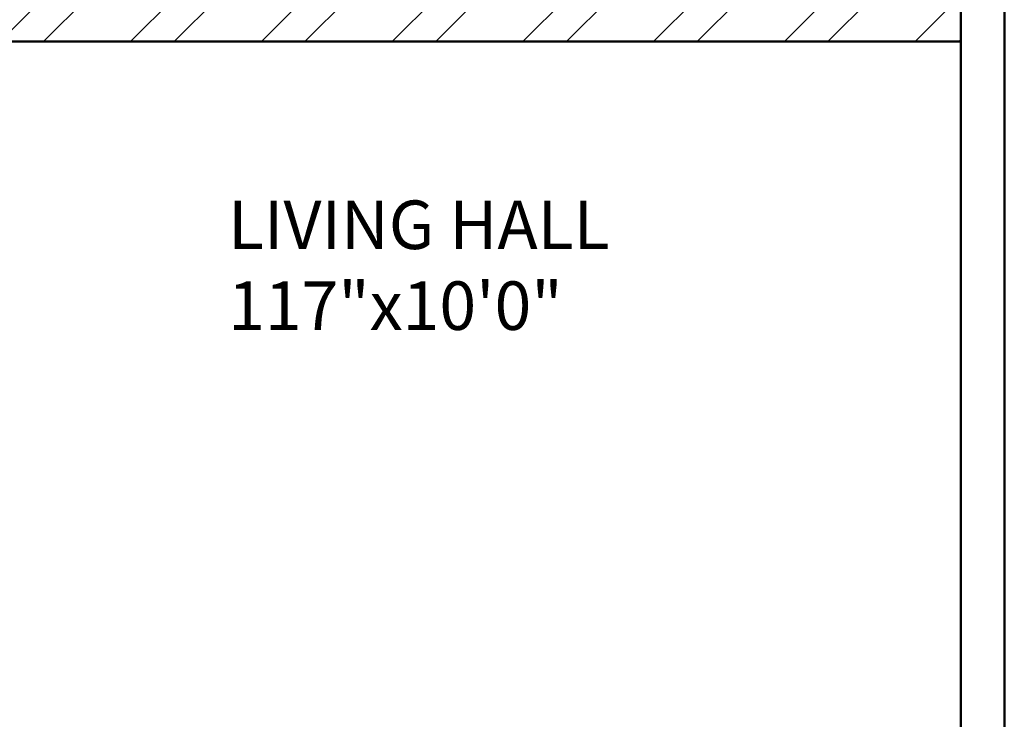
# Model space of a CAD drawing. Units: inches. Extents: x 1901 to 2863, y 888 to 2433.
# Tile 69 of 91: x 2651 to 2753, y 1812 to 1884. Entities that reach past the tile are written whole.
import ezdxf

# ---------------------------------------------------------------- set-up
doc = ezdxf.new("R2010")
doc.units = ezdxf.units.IN
for name, color, linetype, lineweight in [('A-AREA-IDEN', 7, 'Continuous', 18), ('A-WALL', 7, 'Continuous', 50), ('A-WALL-PATT', 8, 'Continuous', 13)]:
    doc.layers.add(name, color=color, linetype=linetype, lineweight=lineweight)
doc.styles.get("Standard").update_dxf_attribs({"font": 'arial.ttf'})

msp = doc.modelspace()

# ---------------------------------------------------------------- hatches: boundary and pattern name
at = {"layer": 'A-WALL-PATT'}
h = msp.add_hatch(dxfattribs=at)
h.set_pattern_fill('ANSI32', color=256)
h.paths.add_polyline_path([(2192.5, 2274.13), (2141.26, 2274.13), (2141.26, 2269.63), (2192.5, 2269.63)])
h.paths.add_polyline_path([(2259.93, 2274.13), (2216.5, 2274.13), (2216.5, 2269.63), (2255.43, 2269.63), (2255.43, 2214.63), (2250.81, 2214.63), (2250.81, 2210.13), (2259.93, 2210.13), (2259.93, 2215.13), (2271.76, 2215.13), (2271.76, 2217.38), (2271.76, 2219.63), (2259.93, 2219.63)])
h.paths.add_polyline_path([(2171.43, 2269.63), (2166.93, 2269.63), (2166.93, 2219.63), (2121.24, 2219.63), (2121.24, 2215.13), (2166.93, 2215.13), (2166.93, 2083.13), (2161.81, 2083.13), (2161.81, 2078.63), (2171.43, 2078.63), (2177, 2078.63), (2177, 2080.88), (2177, 2083.13), (2171.43, 2083.13), (2171.43, 2210.13), (2230.91, 2210.13), (2230.91, 2212.38), (2230.91, 2214.63), (2171.43, 2214.63)])
h.paths.add_polyline_path([(2117.26, 2274.13), (2089.43, 2274.13), (2089.43, 2219.63), (2081.14, 2219.63), (2081.14, 2215.13), (2089.43, 2215.13), (2098, 2215.13), (2098, 2217.38), (2098, 2219.63), (2093.93, 2219.63), (2093.93, 2269.63), (2117.26, 2269.63), (2117.26, 2271.88)])
h.paths.add_polyline_path([(2343.43, 2219.63), (2329.29, 2219.63), (2329.29, 2215.13), (2338.93, 2215.13), (2338.93, 2184.74), (2343.43, 2184.74)])
h.paths.add_polyline_path([(2338.93, 2083.13), (2329.29, 2083.13), (2208.97, 2083.13), (2208.97, 2078.63), (2338.93, 2078.63)])
h.paths.add_polyline_path([(2343.43, 2136.74), (2338.93, 2136.74), (2338.93, 1872.63), (2343.43, 1872.63)])
h.paths.add_polyline_path([(2343.43, 1863.63), (2397.68, 1863.63), (2397.68, 1821.63), (2384.14, 1821.63), (2384.14, 1812.63), (2418.33, 1812.63), (2418.33, 1817.13), (2418.33, 1821.63), (2406.68, 1821.63), (2406.68, 1863.63), (2459.5, 1863.63), (2459.5, 1821.63), (2447.14, 1821.63), (2447.14, 1812.63), (2459.5, 1812.63), (2468.5, 1812.63), (2468.5, 1872.63), (2394.43, 1872.63), (2334.43, 1872.63), (2334.43, 1812.63), (2343.43, 1812.63), (2353.25, 1812.63), (2353.25, 1821.63), (2343.43, 1821.63)])
h.paths.add_polyline_path([(2510.01, 1872.63), (2468.5, 1872.63), (2468.5, 1868.13), (2510.01, 1868.13)])
h.paths.add_polyline_path([(2514.01, 1817.13), (2468.5, 1817.13), (2468.5, 1812.63), (2482.11, 1812.63), (2482.11, 1800.61), (2486.61, 1800.61), (2486.61, 1812.63), (2514.01, 1812.63)])
h.paths.add_polyline_path([(2299.25, 1814.88), (2299.25, 1817.13), (2295.93, 1817.13), (2295.93, 1854.17), (2293.68, 1854.17), (2291.43, 1854.17), (2291.43, 1817.13), (2266.11, 1817.13), (2266.11, 1812.63), (2299.25, 1812.63)])
h.paths.add_polyline_path([(2218.11, 1817.13), (2206.46, 1817.13), (2171.43, 1817.13), (2171.43, 1949.13), (2190.1, 1949.13), (2190.1, 1953.63), (2163.47, 1953.63), (2163.47, 1949.13), (2166.93, 1949.13), (2166.93, 1817.13), (2114.3, 1817.13), (2114.3, 1812.63), (2218.11, 1812.63)])
h.paths.add_polyline_path([(2029.43, 1970.92), (2024.93, 1970.92), (2024.93, 1912.72), (2029.43, 1912.72)])
h.paths.add_polyline_path([(2132.3, 1953.63), (2113.93, 1953.63), (2113.93, 1975.89), (2111.68, 1975.89), (2109.43, 1975.89), (2109.43, 1953.63), (2029.43, 1953.63), (2029.43, 1949.13), (2132.3, 1949.13)])
h.paths.add_polyline_path([(2029.43, 1853.61), (2029.31, 1853.61), (2029.31, 1853.61), (2029.43, 1853.61), (2029.43, 1864.72), (2024.93, 1864.72), (2024.93, 1812.63), (2066.3, 1812.63), (2066.3, 1814.88), (2066.3, 1817.13), (2029.43, 1817.13)])
h.paths.add_polyline_path([(2122.93, 2010.09), (2120.68, 2010.09), (2118.43, 2010.09), (2118.43, 2006.13), (2029.43, 2006.13), (2029.43, 2001.63), (2109.43, 2001.63), (2109.43, 1998.04), (2113.93, 1998.04), (2113.93, 2001.63), (2122.93, 2001.63)])
h.paths.add_polyline_path([(2029.43, 2031.38), (2024.93, 2031.38), (2024.93, 1994.92), (2027.18, 1994.92), (2029.43, 1994.92)])
h.paths.add_polyline_path([(2029.43, 2136.74), (2024.93, 2136.74), (2024.93, 2067.38), (2027.18, 2067.38), (2029.43, 2067.38)])
h.paths.add_polyline_path([(2125.62, 2083.13), (2029.43, 2083.13), (2029.43, 2078.63), (2118.43, 2078.63), (2118.43, 2030.71), (2122.93, 2030.71), (2122.93, 2078.63), (2125.62, 2078.63)])
h.paths.add_polyline_path([(2029.43, 2215.13), (2040.47, 2215.13), (2040.47, 2217.38), (2040.47, 2219.63), (2024.93, 2219.63), (2024.93, 2184.74), (2029.43, 2184.74), (2029.43, 2187.78)])
h.paths.add_polyline_path([(2686.43, 2274.13), (2659.28, 2274.13), (2659.28, 2269.63), (2681.93, 2269.63), (2681.93, 2219.63), (2676.82, 2219.63), (2676.82, 2215.13), (2681.93, 2215.13), (2697.01, 2215.13), (2697.01, 2217.38), (2697.01, 2219.63), (2686.43, 2219.63)])
h.paths.add_polyline_path([(2609.93, 2269.63), (2635.28, 2269.63), (2635.28, 2274.13), (2571.43, 2274.13), (2571.43, 2269.63), (2605.43, 2269.63), (2605.43, 2214.63), (2549.1, 2214.63), (2549.1, 2210.13), (2605.43, 2210.13), (2605.43, 2083.13), (2601.01, 2083.13), (2601.01, 2080.88), (2601.01, 2078.63), (2609.93, 2078.63), (2616.16, 2078.63), (2616.16, 2080.88), (2616.16, 2083.13), (2609.93, 2083.13), (2609.93, 2215.13), (2651.46, 2215.13), (2651.46, 2217.38), (2651.46, 2219.63), (2609.93, 2219.63)])
h.paths.add_polyline_path([(2521.43, 2269.63), (2547.43, 2269.63), (2547.43, 2271.88), (2547.43, 2274.13), (2516.93, 2274.13), (2516.93, 2219.63), (2506.41, 2219.63), (2506.41, 2215.13), (2516.93, 2215.13), (2516.93, 2210.13), (2525.4, 2210.13), (2525.4, 2212.38), (2525.4, 2214.63), (2521.43, 2214.63)])
h.paths.add_polyline_path([(2456.01, 2219.63), (2439.43, 2219.63), (2439.43, 2187.89), (2443.93, 2187.89), (2443.93, 2215.13), (2456.01, 2215.13)])
h.paths.add_polyline_path([(2752.93, 2219.63), (2739.48, 2219.63), (2739.48, 2215.13), (2748.43, 2215.13), (2748.43, 2187.89), (2752.93, 2187.89)])
h.paths.add_polyline_path([(2752.93, 2139.89), (2748.43, 2139.89), (2748.43, 2083.13), (2648.42, 2083.13), (2648.42, 2078.63), (2654.93, 2078.63), (2654.93, 2039.44), (2659.43, 2039.44), (2659.43, 2078.63), (2748.43, 2078.63), (2748.43, 2063.43), (2752.93, 2063.43)])
h.paths.add_polyline_path([(2752.93, 2010.63), (2659.43, 2010.63), (2659.43, 2015.65), (2654.93, 2015.65), (2654.93, 2010.63), (2605.43, 2010.63), (2605.43, 1920.97), (2609.93, 1920.97), (2609.93, 2006.13), (2748.43, 2006.13), (2748.43, 1982.47), (2752.93, 1982.47)])
h.paths.add_polyline_path([(2752.93, 2027.43), (2748.43, 2027.43), (2748.43, 2010.63), (2752.93, 2010.63)])
h.paths.add_polyline_path([(2748.43, 1886.13), (2609.93, 1886.13), (2609.93, 1889.72), (2605.43, 1889.72), (2605.43, 1861.26), (2609.93, 1861.26), (2609.93, 1881.63), (2748.43, 1881.63)])
h.paths.add_polyline_path([(2456.86, 2228.83), (2498.4, 2228.83), (2498.4, 2247.49), (2456.86, 2247.49)], flags=9)
h.paths.add_polyline_path([(2038.6, 2237.42), (2080.17, 2237.42), (2080.17, 2256.08), (2038.6, 2256.08)], flags=9)
h.paths.add_polyline_path([(2292.01, 1062.39), (2539.93, 1062.39), (2539.93, 1099.49), (2292.01, 1099.49)], flags=9)
h.paths.add_polyline_path([(2424.91, 1832.25), (2448.51, 1832.25), (2448.51, 1846.68), (2424.91, 1846.68)], flags=25)
h.paths.add_polyline_path([(2359.08, 1832.25), (2382.68, 1832.25), (2382.68, 1846.68), (2359.08, 1846.68)], flags=25)
h.paths.add_polyline_path([(2352.9, 1684.8), (2367.54, 1684.8), (2367.54, 1697.17), (2352.9, 1697.17)], flags=9)
h.paths.add_polyline_path([(2079.29, 1755.83), (2169.02, 1755.83), (2169.02, 1774.37), (2079.29, 1774.37)], flags=9)
h.paths.add_polyline_path([(2404.09, 1373.86), (2404.09, 1463.59), (2385.54, 1463.59), (2385.54, 1373.86)], flags=9)
h.paths.add_polyline_path([(2268.09, 2236.37), (2309.64, 2236.37), (2309.64, 2255.03), (2268.09, 2255.03)], flags=9)
h.paths.add_polyline_path([(2575.96, 1700.95), (2665.7, 1700.95), (2665.7, 1719.5), (2575.96, 1719.5)], flags=9)
h.paths.add_polyline_path([(2302.96, 1878.47), (2329.52, 1878.47), (2329.52, 1888.78), (2302.96, 1888.78)], flags=9)
h.paths.add_polyline_path([(2097.42, 2240.58), (2126.57, 2240.58), (2126.57, 2259.23), (2097.42, 2259.23)], flags=9)
h.paths.add_polyline_path([(2208.72, 2246.12), (2237.88, 2246.12), (2237.88, 2264.78), (2208.72, 2264.78)], flags=9)
h.paths.add_polyline_path([(2038.15, 1925.96), (2076.99, 1925.96), (2076.99, 1944.62), (2038.15, 1944.62)], flags=9)
h.paths.add_polyline_path([(2239.14, 1926.67), (2288.46, 1926.67), (2288.46, 1945.33), (2239.14, 1945.33)], flags=9)
h.paths.add_polyline_path([(2175.43, 2007.33), (2212.36, 2007.33), (2212.36, 2025.99), (2175.43, 2025.99)], flags=9)
h.paths.add_polyline_path([(2225.03, 2091.79), (2263.87, 2091.79), (2263.87, 2110.45), (2225.03, 2110.45)], flags=9)
h.paths.add_polyline_path([(2035.4, 2098.48), (2074.24, 2098.48), (2074.24, 2117.14), (2035.4, 2117.14)], flags=9)
h.paths.add_polyline_path([(2050.1, 2029.21), (2083.26, 2029.21), (2083.26, 2047.87), (2050.1, 2047.87)], flags=9)
h.paths.add_polyline_path([(2069.68, 1956.72), (2098.83, 1956.72), (2098.83, 1975.38), (2069.68, 1975.38)], flags=25)
h.paths.add_polyline_path([(2328.62, 1753.34), (2361.66, 1753.34), (2361.66, 1771.99), (2328.62, 1771.99)], flags=9)
h.paths.add_polyline_path([(2395.16, 2060.89), (2395.16, 2140.65), (2378.68, 2140.65), (2378.68, 2060.89)], flags=9)
h.paths.add_polyline_path([(2463.73, 2059.02), (2492.89, 2059.02), (2492.89, 2077.68), (2463.73, 2077.68)], flags=9)
h.paths.add_polyline_path([(2458.03, 2181.54), (2496.87, 2181.54), (2496.87, 2200.19), (2458.03, 2200.19)], flags=9)
h.paths.add_polyline_path([(2527.58, 2243.07), (2556.73, 2243.07), (2556.73, 2261.73), (2527.58, 2261.73)], flags=9)
h.paths.add_polyline_path([(2694.46, 2232.77), (2736.03, 2232.77), (2736.03, 2251.42), (2694.46, 2251.42)], flags=9)
h.paths.add_polyline_path([(2637.82, 2249.22), (2666.98, 2249.22), (2666.98, 2267.88), (2637.82, 2267.88)], flags=9)
h.paths.add_polyline_path([(2623.69, 2183.54), (2662.53, 2183.54), (2662.53, 2202.2), (2623.69, 2202.2)], flags=9)
h.paths.add_polyline_path([(2691.97, 2021.5), (2725.12, 2021.5), (2725.12, 2040.16), (2691.97, 2040.16)], flags=9)
h.paths.add_polyline_path([(2621.04, 1975.91), (2662.34, 1975.91), (2662.34, 1994.57), (2621.04, 1994.57)], flags=25)
h.paths.add_polyline_path([(2479.03, 1927.62), (2519.84, 1927.62), (2519.84, 1946.28), (2479.03, 1946.28)], flags=9)
h.paths.add_polyline_path([(2670.94, 1849.08), (2716.01, 1849.08), (2716.01, 1867.73), (2670.94, 1867.73)], flags=9)
h.paths.add_polyline_path([(2523.61, 1782.96), (2550.17, 1782.96), (2550.17, 1793.26), (2523.61, 1793.26)], flags=9)
h.paths.add_polyline_path([(2450.84, 1207.33), (2492.39, 1207.33), (2492.39, 1225.99), (2450.84, 1225.99)], flags=9)
h.paths.add_polyline_path([(2527.75, 1203.84), (2556.91, 1203.84), (2556.91, 1222.5), (2527.75, 1222.5)], flags=9)
h.paths.add_polyline_path([(2639.11, 1207.2), (2668.27, 1207.2), (2668.27, 1225.86), (2639.11, 1225.86)], flags=9)
h.paths.add_polyline_path([(2692.59, 1218.97), (2734.17, 1218.97), (2734.17, 1237.62), (2692.59, 1237.62)], flags=9)
h.paths.add_polyline_path([(2669.27, 1366.33), (2708.11, 1366.33), (2708.11, 1384.99), (2669.27, 1384.99)], flags=9)
h.paths.add_polyline_path([(2463.31, 1358.03), (2502.15, 1358.03), (2502.15, 1376.69), (2463.31, 1376.69)], flags=9)
h.paths.add_polyline_path([(2494.72, 1449.96), (2531.65, 1449.96), (2531.65, 1468.62), (2494.72, 1468.62)], flags=9)
h.paths.add_polyline_path([(2675.57, 1422.16), (2708.72, 1422.16), (2708.72, 1440.81), (2675.57, 1440.81)], flags=9)
h.paths.add_polyline_path([(2685.63, 1493.89), (2714.79, 1493.89), (2714.79, 1512.55), (2685.63, 1512.55)], flags=9)
h.paths.add_polyline_path([(2686.8, 1529.91), (2725.65, 1529.91), (2725.65, 1548.57), (2686.8, 1548.57)], flags=9)
h.paths.add_polyline_path([(2503.65, 1537.99), (2552.97, 1537.99), (2552.97, 1556.65), (2503.65, 1556.65)], flags=9)
h.paths.add_polyline_path([(2291.71, 1643.5), (2318.28, 1643.5), (2318.28, 1653.81), (2291.71, 1653.81)], flags=9)
h.paths.add_polyline_path([(2450.63, 1610.52), (2477.19, 1610.52), (2477.19, 1620.82), (2450.63, 1620.82)], flags=9)
h.paths.add_polyline_path([(2359.99, 1551.81), (2422.25, 1551.81), (2422.25, 1562.12), (2359.99, 1562.12)], flags=9)
h.paths.add_polyline_path([(2280.11, 1249.01), (2321.65, 1249.01), (2321.65, 1267.66), (2280.11, 1267.66)], flags=9)
h.paths.add_polyline_path([(2164.06, 1274.23), (2193.22, 1274.23), (2193.22, 1292.89), (2164.06, 1292.89)], flags=9)
h.paths.add_polyline_path([(2118.21, 1277.69), (2151.25, 1277.69), (2151.25, 1296.35), (2118.21, 1296.35)], flags=9)
h.paths.add_polyline_path([(2031.95, 1268.53), (2073.52, 1268.53), (2073.52, 1287.19), (2031.95, 1287.19)], flags=9)
h.paths.add_polyline_path([(2050.2, 1409.08), (2089.04, 1409.08), (2089.04, 1427.74), (2050.2, 1427.74)], flags=9)
h.paths.add_polyline_path([(2243.74, 1421.03), (2282.58, 1421.03), (2282.58, 1439.69), (2243.74, 1439.69)], flags=9)
h.paths.add_polyline_path([(2190.75, 1509.77), (2231.56, 1509.77), (2231.56, 1528.43), (2190.75, 1528.43)], flags=9)
h.paths.add_polyline_path([(2058.39, 1475.42), (2091.55, 1475.42), (2091.55, 1494.07), (2058.39, 1494.07)], flags=9)
h.paths.add_polyline_path([(2062.45, 1553.09), (2091.6, 1553.09), (2091.6, 1571.75), (2062.45, 1571.75)], flags=9)
h.paths.add_polyline_path([(2219.52, 1590.37), (2266.15, 1590.37), (2266.15, 1609.02), (2219.52, 1609.02)], flags=9)
h.paths.add_polyline_path([(2041.07, 1584.19), (2079.91, 1584.19), (2079.91, 1602.85), (2041.07, 1602.85)], flags=9)
h = msp.add_hatch(dxfattribs=at)
h.set_pattern_fill('ANSI32', color=256)
h.paths.add_polyline_path([(2443.93, 2139.89), (2439.43, 2139.89), (2439.43, 2069.35), (2441.68, 2069.35), (2443.93, 2069.35), (2443.93, 2078.63), (2521.93, 2078.63), (2521.93, 2075.07), (2524.18, 2075.07), (2526.43, 2075.07), (2526.43, 2078.63), (2571.75, 2078.63), (2571.75, 2080.88), (2571.75, 2083.13), (2443.93, 2083.13)])
h.paths.add_polyline_path([(2526.43, 2054.63), (2524.18, 2054.63), (2521.93, 2054.63), (2521.93, 2030.63), (2443.93, 2030.63), (2443.93, 2045.35), (2439.43, 2045.35), (2439.43, 1983.87), (2443.93, 1983.87), (2443.93, 2026.13), (2521.93, 2026.13), (2526.43, 2026.13)])
h.paths.add_polyline_path([(2443.93, 1923.87), (2439.43, 1923.87), (2439.43, 1872.63), (2443.93, 1872.63)])
h.paths.add_polyline_path([(2636.23, 1766.13), (2609.93, 1766.13), (2609.93, 1779.79), (2605.43, 1779.79), (2605.43, 1766.13), (2486.61, 1766.13), (2486.61, 1770.67), (2482.11, 1770.67), (2482.11, 1766.13), (2482.11, 1761.63), (2636.23, 1761.63), (2636.23, 1763.88)])
h.paths.add_polyline_path([(2519.54, 1663.38), (2519.54, 1665.63), (2494.93, 1665.63), (2481.83, 1665.63), (2481.83, 1663.38), (2481.83, 1661.13), (2490.43, 1661.13), (2490.43, 1640.16), (2494.93, 1640.16), (2494.93, 1661.13), (2519.54, 1661.13)])
h.paths.add_polyline_path([(2443.93, 1712.13), (2443.93, 1716.63), (2414.46, 1716.63), (2414.46, 1712.13), (2439.43, 1712.13), (2439.43, 1545.51), (2443.93, 1545.51), (2443.93, 1661.13), (2448.47, 1661.13), (2448.47, 1665.63), (2443.93, 1665.63)])
h.paths.add_polyline_path([(2343.43, 1712.13), (2365.52, 1712.13), (2365.52, 1714.38), (2365.52, 1716.63), (2333.87, 1716.63), (2333.87, 1714.38), (2333.87, 1712.13), (2338.93, 1712.13), (2338.93, 1575.63), (2338.93, 1545.51), (2343.43, 1545.51), (2343.43, 1547.51), (2343.43, 1580.13)])
h.paths.add_polyline_path([(2752.93, 1665.63), (2579.54, 1665.63), (2579.54, 1661.13), (2615.93, 1661.13), (2615.93, 1529.13), (2598.93, 1529.13), (2598.93, 1524.63), (2623.13, 1524.63), (2623.13, 1526.88), (2623.13, 1529.13), (2620.43, 1529.13), (2620.43, 1661.13), (2748.43, 1661.13), (2748.43, 1633.5), (2752.93, 1633.5)])
h.paths.add_polyline_path([(2752.93, 1419.93), (2748.43, 1419.93), (2748.43, 1400.13), (2659.43, 1400.13), (2659.43, 1444.33), (2657.18, 1444.33), (2654.93, 1444.33), (2654.93, 1400.13), (2643.65, 1400.13), (2643.65, 1395.63), (2748.43, 1395.63), (2748.43, 1364.04), (2752.93, 1364.04)])
h.paths.add_polyline_path([(2752.93, 1492.88), (2748.43, 1492.88), (2748.43, 1476.63), (2667.43, 1476.63), (2667.43, 1479.71), (2665.18, 1479.71), (2662.93, 1479.71), (2662.93, 1476.63), (2654.93, 1476.63), (2654.93, 1469.54), (2659.43, 1469.54), (2659.43, 1472.13), (2748.43, 1472.13), (2748.43, 1455.93), (2752.93, 1455.93)])
h.paths.add_polyline_path([(2752.93, 1304.04), (2748.43, 1304.04), (2748.43, 1263.63), (2738.66, 1263.63), (2738.66, 1259.13), (2752.93, 1259.13)])
h.paths.add_polyline_path([(2685.93, 1259.13), (2695.49, 1259.13), (2695.49, 1261.38), (2695.49, 1263.63), (2677.84, 1263.63), (2677.84, 1261.38), (2677.84, 1259.13), (2681.43, 1259.13), (2681.43, 1203.63), (2653.28, 1203.63), (2653.28, 1199.13), (2685.93, 1199.13), (2685.93, 1203.63)])
h.paths.add_polyline_path([(2609.43, 1395.63), (2611.85, 1395.63), (2611.85, 1400.13), (2598.89, 1400.13), (2598.89, 1397.88), (2598.89, 1395.63), (2604.93, 1395.63), (2604.93, 1268.13), (2554.73, 1268.13), (2554.73, 1265.88), (2554.73, 1263.63), (2604.93, 1263.63), (2604.93, 1203.63), (2571.31, 1203.63), (2571.31, 1199.13), (2604.93, 1199.13), (2629.28, 1199.13), (2629.28, 1201.38), (2629.28, 1203.63), (2609.43, 1203.63), (2609.43, 1258.63), (2609.43, 1259.13), (2654.8, 1259.13), (2654.8, 1263.63), (2609.43, 1263.63)])
h.paths.add_polyline_path([(2443.93, 1304.04), (2439.43, 1304.04), (2439.43, 1259.13), (2443.93, 1259.13), (2456.16, 1259.13), (2456.16, 1261.38), (2456.16, 1263.63), (2443.93, 1263.63)])
h.paths.add_polyline_path([(2525.43, 1263.63), (2531.78, 1263.63), (2531.78, 1268.13), (2520.93, 1268.13), (2520.93, 1263.63), (2511.41, 1263.63), (2511.41, 1259.13), (2520.93, 1259.13), (2520.93, 1199.13), (2547.31, 1199.13), (2547.31, 1201.38), (2547.31, 1203.63), (2525.43, 1203.63)])
h.paths.add_polyline_path([(2443.93, 1434.84), (2439.43, 1434.84), (2439.43, 1364.04), (2441.68, 1364.04), (2443.93, 1364.04)])
h.paths.add_polyline_path([(2567.13, 1400.13), (2443.93, 1400.13), (2443.93, 1395.63), (2567.13, 1395.63)])
h.paths.add_polyline_path([(2443.93, 1545.51), (2439.43, 1545.51), (2439.43, 1494.84), (2443.93, 1494.84)])
h.paths.add_polyline_path([(2494.93, 1553.35), (2492.68, 1553.35), (2490.43, 1553.35), (2490.43, 1524.63), (2494.93, 1524.63), (2525.94, 1524.63), (2525.94, 1526.88), (2525.94, 1529.13), (2494.93, 1529.13)])
h.paths.add_polyline_path([(2752.93, 1573.5), (2748.43, 1573.5), (2748.43, 1529.13), (2657.76, 1529.13), (2657.76, 1524.63), (2662.93, 1524.63), (2662.93, 1498.63), (2667.43, 1498.63), (2667.43, 1524.63), (2748.43, 1524.63), (2748.43, 1516.88), (2752.93, 1516.88)])
h.paths.add_polyline_path([(2038.6, 2237.42), (2080.17, 2237.42), (2080.17, 2256.08), (2038.6, 2256.08)], flags=9)
h.paths.add_polyline_path([(2292.01, 1062.39), (2539.93, 1062.39), (2539.93, 1099.49), (2292.01, 1099.49)], flags=9)
h.paths.add_polyline_path([(2424.91, 1832.25), (2448.51, 1832.25), (2448.51, 1846.68), (2424.91, 1846.68)], flags=9)
h.paths.add_polyline_path([(2359.08, 1832.25), (2382.68, 1832.25), (2382.68, 1846.68), (2359.08, 1846.68)], flags=9)
h.paths.add_polyline_path([(2352.9, 1684.8), (2367.54, 1684.8), (2367.54, 1697.17), (2352.9, 1697.17)], flags=9)
h.paths.add_polyline_path([(2079.29, 1755.83), (2169.02, 1755.83), (2169.02, 1774.37), (2079.29, 1774.37)], flags=9)
h.paths.add_polyline_path([(2404.09, 1373.86), (2404.09, 1463.59), (2385.54, 1463.59), (2385.54, 1373.86)], flags=9)
h.paths.add_polyline_path([(2268.09, 2236.37), (2309.64, 2236.37), (2309.64, 2255.03), (2268.09, 2255.03)], flags=9)
h.paths.add_polyline_path([(2575.96, 1700.95), (2665.7, 1700.95), (2665.7, 1719.5), (2575.96, 1719.5)], flags=9)
h.paths.add_polyline_path([(2302.96, 1878.47), (2329.52, 1878.47), (2329.52, 1888.78), (2302.96, 1888.78)], flags=9)
h.paths.add_polyline_path([(2097.42, 2240.58), (2126.57, 2240.58), (2126.57, 2259.23), (2097.42, 2259.23)], flags=9)
h.paths.add_polyline_path([(2208.72, 2246.12), (2237.88, 2246.12), (2237.88, 2264.78), (2208.72, 2264.78)], flags=9)
h.paths.add_polyline_path([(2038.15, 1925.96), (2076.99, 1925.96), (2076.99, 1944.62), (2038.15, 1944.62)], flags=9)
h.paths.add_polyline_path([(2239.14, 1926.67), (2288.46, 1926.67), (2288.46, 1945.33), (2239.14, 1945.33)], flags=9)
h.paths.add_polyline_path([(2175.43, 2007.33), (2212.36, 2007.33), (2212.36, 2025.99), (2175.43, 2025.99)], flags=9)
h.paths.add_polyline_path([(2225.03, 2091.79), (2263.87, 2091.79), (2263.87, 2110.45), (2225.03, 2110.45)], flags=9)
h.paths.add_polyline_path([(2035.4, 2098.48), (2074.24, 2098.48), (2074.24, 2117.14), (2035.4, 2117.14)], flags=9)
h.paths.add_polyline_path([(2050.1, 2029.21), (2083.26, 2029.21), (2083.26, 2047.87), (2050.1, 2047.87)], flags=9)
h.paths.add_polyline_path([(2069.68, 1956.72), (2098.83, 1956.72), (2098.83, 1975.38), (2069.68, 1975.38)], flags=9)
h.paths.add_polyline_path([(2328.62, 1753.34), (2361.66, 1753.34), (2361.66, 1771.99), (2328.62, 1771.99)], flags=9)
h.paths.add_polyline_path([(2395.16, 2060.89), (2395.16, 2140.65), (2378.68, 2140.65), (2378.68, 2060.89)], flags=9)
h.paths.add_polyline_path([(2463.73, 2059.02), (2492.89, 2059.02), (2492.89, 2077.68), (2463.73, 2077.68)], flags=9)
h.paths.add_polyline_path([(2458.03, 2181.54), (2496.87, 2181.54), (2496.87, 2200.19), (2458.03, 2200.19)], flags=9)
h.paths.add_polyline_path([(2456.86, 2228.83), (2498.4, 2228.83), (2498.4, 2247.49), (2456.86, 2247.49)], flags=9)
h.paths.add_polyline_path([(2527.58, 2243.07), (2556.73, 2243.07), (2556.73, 2261.73), (2527.58, 2261.73)], flags=9)
h.paths.add_polyline_path([(2694.46, 2232.77), (2736.03, 2232.77), (2736.03, 2251.42), (2694.46, 2251.42)], flags=9)
h.paths.add_polyline_path([(2637.82, 2249.22), (2666.98, 2249.22), (2666.98, 2267.88), (2637.82, 2267.88)], flags=9)
h.paths.add_polyline_path([(2623.69, 2183.54), (2662.53, 2183.54), (2662.53, 2202.2), (2623.69, 2202.2)], flags=9)
h.paths.add_polyline_path([(2691.97, 2021.5), (2725.12, 2021.5), (2725.12, 2040.16), (2691.97, 2040.16)], flags=9)
h.paths.add_polyline_path([(2621.04, 1975.91), (2662.34, 1975.91), (2662.34, 1994.57), (2621.04, 1994.57)], flags=9)
h.paths.add_polyline_path([(2479.03, 1927.62), (2519.84, 1927.62), (2519.84, 1946.28), (2479.03, 1946.28)], flags=9)
h.paths.add_polyline_path([(2670.94, 1849.08), (2716.01, 1849.08), (2716.01, 1867.73), (2670.94, 1867.73)], flags=9)
h.paths.add_polyline_path([(2523.61, 1782.96), (2550.17, 1782.96), (2550.17, 1793.26), (2523.61, 1793.26)], flags=9)
h.paths.add_polyline_path([(2450.84, 1207.33), (2492.39, 1207.33), (2492.39, 1225.99), (2450.84, 1225.99)], flags=9)
h.paths.add_polyline_path([(2527.75, 1203.84), (2556.91, 1203.84), (2556.91, 1222.5), (2527.75, 1222.5)], flags=9)
h.paths.add_polyline_path([(2639.11, 1207.2), (2668.27, 1207.2), (2668.27, 1225.86), (2639.11, 1225.86)], flags=9)
h.paths.add_polyline_path([(2692.59, 1218.97), (2734.17, 1218.97), (2734.17, 1237.62), (2692.59, 1237.62)], flags=9)
h.paths.add_polyline_path([(2669.27, 1366.33), (2708.11, 1366.33), (2708.11, 1384.99), (2669.27, 1384.99)], flags=25)
h.paths.add_polyline_path([(2463.31, 1358.03), (2502.15, 1358.03), (2502.15, 1376.69), (2463.31, 1376.69)], flags=9)
h.paths.add_polyline_path([(2494.72, 1449.96), (2531.65, 1449.96), (2531.65, 1468.62), (2494.72, 1468.62)], flags=9)
h.paths.add_polyline_path([(2675.57, 1422.16), (2708.72, 1422.16), (2708.72, 1440.81), (2675.57, 1440.81)], flags=25)
h.paths.add_polyline_path([(2685.63, 1493.89), (2714.79, 1493.89), (2714.79, 1512.55), (2685.63, 1512.55)], flags=9)
h.paths.add_polyline_path([(2686.8, 1529.91), (2725.65, 1529.91), (2725.65, 1548.57), (2686.8, 1548.57)], flags=25)
h.paths.add_polyline_path([(2503.65, 1537.99), (2552.97, 1537.99), (2552.97, 1556.65), (2503.65, 1556.65)], flags=9)
h.paths.add_polyline_path([(2291.71, 1643.5), (2318.28, 1643.5), (2318.28, 1653.81), (2291.71, 1653.81)], flags=9)
h.paths.add_polyline_path([(2450.63, 1610.52), (2477.19, 1610.52), (2477.19, 1620.82), (2450.63, 1620.82)], flags=9)
h.paths.add_polyline_path([(2359.99, 1551.81), (2422.25, 1551.81), (2422.25, 1562.12), (2359.99, 1562.12)], flags=9)
h.paths.add_polyline_path([(2280.11, 1249.01), (2321.65, 1249.01), (2321.65, 1267.66), (2280.11, 1267.66)], flags=9)
h.paths.add_polyline_path([(2164.06, 1274.23), (2193.22, 1274.23), (2193.22, 1292.89), (2164.06, 1292.89)], flags=9)
h.paths.add_polyline_path([(2118.21, 1277.69), (2151.25, 1277.69), (2151.25, 1296.35), (2118.21, 1296.35)], flags=9)
h.paths.add_polyline_path([(2031.95, 1268.53), (2073.52, 1268.53), (2073.52, 1287.19), (2031.95, 1287.19)], flags=9)
h.paths.add_polyline_path([(2050.2, 1409.08), (2089.04, 1409.08), (2089.04, 1427.74), (2050.2, 1427.74)], flags=9)
h.paths.add_polyline_path([(2243.74, 1421.03), (2282.58, 1421.03), (2282.58, 1439.69), (2243.74, 1439.69)], flags=9)
h.paths.add_polyline_path([(2190.75, 1509.77), (2231.56, 1509.77), (2231.56, 1528.43), (2190.75, 1528.43)], flags=9)
h.paths.add_polyline_path([(2058.39, 1475.42), (2091.55, 1475.42), (2091.55, 1494.07), (2058.39, 1494.07)], flags=9)
h.paths.add_polyline_path([(2062.45, 1553.09), (2091.6, 1553.09), (2091.6, 1571.75), (2062.45, 1571.75)], flags=9)
h.paths.add_polyline_path([(2219.52, 1590.37), (2266.15, 1590.37), (2266.15, 1609.02), (2219.52, 1609.02)], flags=9)
h.paths.add_polyline_path([(2041.07, 1584.19), (2079.91, 1584.19), (2079.91, 1602.85), (2041.07, 1602.85)], flags=9)

# ---------------------------------------------------------------- linework, layer by layer
at = {"layer": 'A-WALL'}
for p, q in [((2752.93, 2219.63), (2752.93, 1812.63)), ((2748.43, 2006.13), (2748.43, 1817.13)), ((2609.93, 1881.63), (2748.43, 1881.63)), ((2748.43, 1817.13), (2748.43, 1766.13)), ((2752.93, 1761.63), (2752.93, 1812.63))]:
    msp.add_line(p, q, dxfattribs=at)

# ---------------------------------------------------------------- texts
at = {"layer": 'A-AREA-IDEN', "insert": (2672.95, 1865.25), "char_height": 5, "attachment_point": 1}
msp.add_mtext_dynamic_manual_height_columns('LIVING HALL\\P117"x10\'0"', width=172.3647, gutter_width=12.5, heights=[0], dxfattribs=at)

doc.saveas('drawing.dxf')
